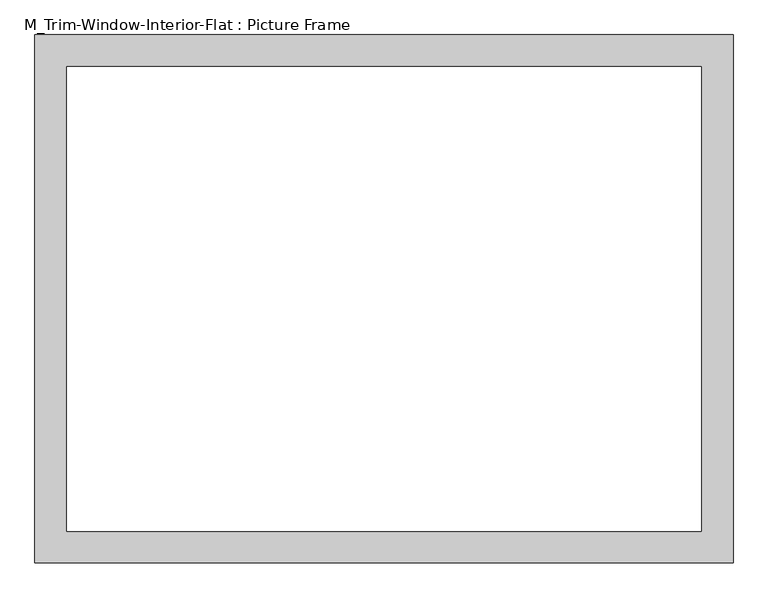
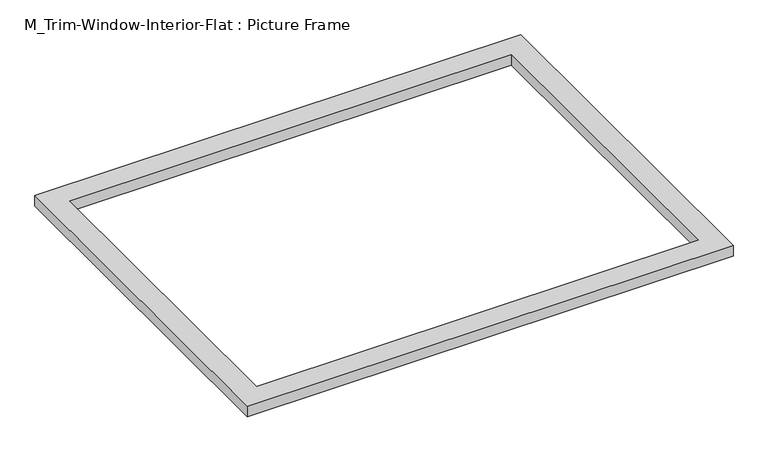
"""IFC4 building model written with IfcOpenShell, lengths in millimetres: proxy geometry, M_Trim-Window-Interior-Flat : Picture Frame."""

from ifc_helpers import new_model, si_unit, origin, origin_with_axes, place, context, project, spatial, polyline, outline, extrude, source, transform, mapped, element, save


def m_trim_window_interior_flat_picture_frame_7d12f20c(model_context):
    return source(origin(), model_context, "Body", "SweptSolid", [
        extrude(outline(polyline([(656.9, 47.3), (656.9, -947.3), (-656.9, -947.3), (-656.9, 47.3), (656.9, 47.3)]), holes=[polyline([(596.9, -12.7), (-596.9, -12.7), (-596.9, -887.3), (596.9, -887.3), (596.9, -12.7)])]), origin_with_axes(), (0.0, 0.0, 1.0), 30.0),
    ])


if __name__ == "__main__":
    model = new_model("IFC4")
    model_context = context("Model", 3, world=origin())
    ifc_project = project(units=[si_unit("LENGTHUNIT", "METRE", prefix="MILLI")], contexts=[model_context])
    site = spatial("IfcSite", under=ifc_project)
    building = spatial("IfcBuilding", under=site)
    placement = place(None, origin())
    m_trim_window_interior_flat_picture_frame_shape = m_trim_window_interior_flat_picture_frame_7d12f20c(model_context)
    element("IfcBuildingElementProxy", 1, Name="M_Trim-Window-Interior-Flat : Picture Frame", ObjectType="M_Trim-Window-Interior-Flat : Picture Frame", at=placement, inside=building, context=model_context, shape_type="MappedRepresentation", body=[
        mapped(m_trim_window_interior_flat_picture_frame_shape, transform((0.0, 0.0, 0.0), x_axis=(1.0, 0.0, 0.0), y_axis=(0.0, 1.0, 0.0), z_axis=(0.0, 0.0, 1.0))),
    ])
    save(model, "model.ifc")

# Revit data of these elements
# Type "M_Trim-Window-Interior-Flat : Picture Frame"
#   Trim Thickness_Picture Frame = 0' - 1.1811"
#   Trim Width = 0' - 2.3622"
#   Trim Thickness_with Sill = 0' - 0.7874"
#   Sill Thickness = 0' - 1.1811"
#   Opening Width [instance default] = 1' - 11.62205"
#   Opening Height [instance default] = 2' - 11.43307"
#   Default Elevation = 3' - 11.24409"
#   Sill = no
#   Picture Frame = yes
#   Trim Material [instance default] = none
# Element 1 (IfcBuildingElementProxy, "M_Trim-Window-Interior-Flat : Picture Frame")
#   Opening Width = 4' - 0"
#   Trim Material = Wood - Stained
#   Materials on its faces: "Wood - Stained"
# Materials
#   "Wood - Stained": class "Wood", colour RGB 227 170 128, transparency 0, Cost = 0
